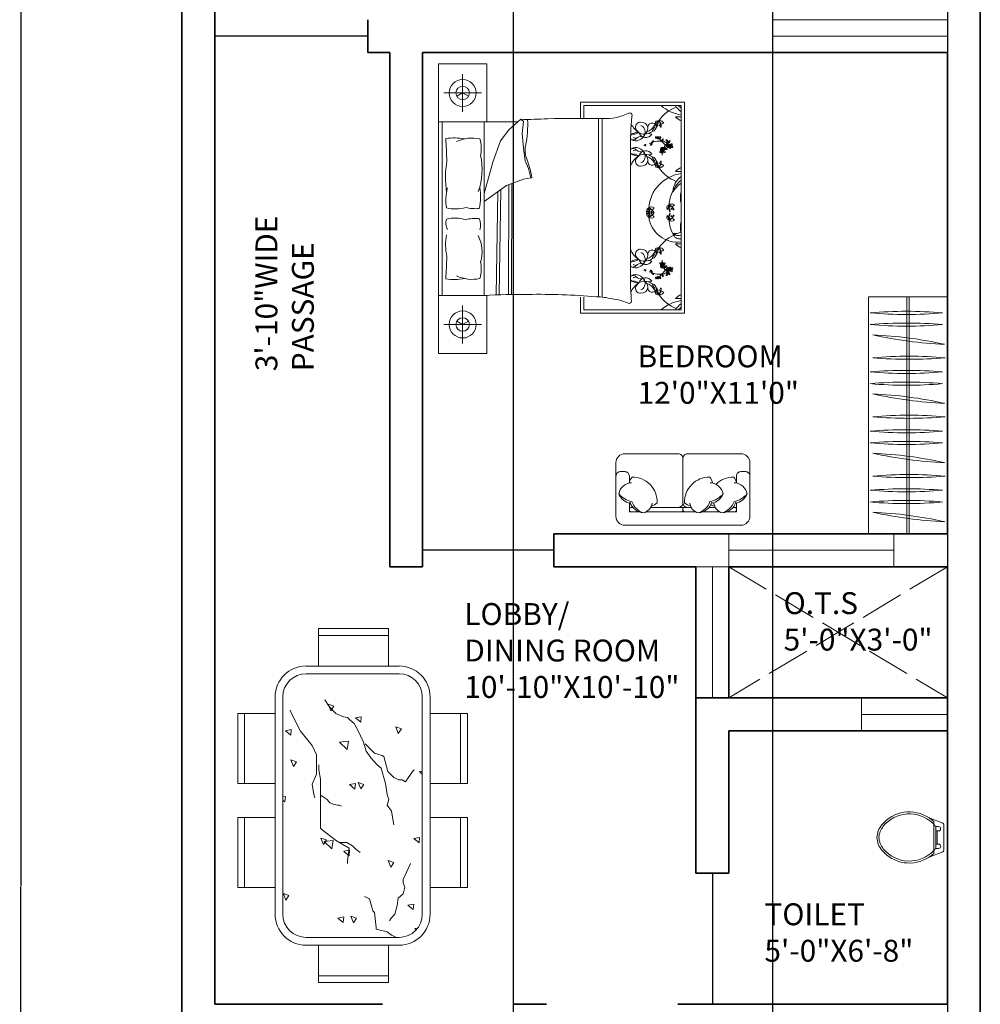
# Model space of a CAD drawing. Units: inches. Extents: x -16 to 587, y -783 to 64.
# Tile 13 of 14: x 279 to 543, y -392 to -122. Entities that reach past the tile are written whole.
import ezdxf

# ---------------------------------------------------------------- set-up
doc = ezdxf.new("R2010")
doc.units = ezdxf.units.IN
doc.header["$MEASUREMENT"] = 0
doc.linetypes.add('ACAD_ISO02W100', pattern=[15, 12, -3])
for name, color, linetype, lineweight in [('A-ANNO-DIMS', 2, 'Continuous', 18), ('A-AREA-IDEN', 7, 'Continuous', 18), ('A-DOOR', 3, 'Continuous', 25), ('A-FLOR-FIXT', 9, 'Continuous', 18), ('A-FLOR-OPEN', 8, 'ACAD_ISO02W100', 13), ('A-FURN', 8, 'Continuous', 18), ('A-GLAZ', 4, 'Continuous', 18), ('A-WALL', 7, 'Continuous', 35)]:
    doc.layers.add(name, color=color, linetype=linetype, lineweight=lineweight)
doc.styles.get("Standard").update_dxf_attribs({"font": 'arial.ttf'})
doc.dimstyles.get("Standard").update_dxf_attribs({"dimtxt": 0.18, "dimasz": 0.18, "dimexe": 0.18, "dimexo": 0.0625, "dimgap": 0.09, "dimtad": 0, "dimtih": 1, "dimtoh": 1, "dimdec": 0, "dimzin": 0, "dimdsep": 46, "dimlunit": 3, "dimtxsty": 'Standard', "dimcen": 0.09, "dimadec": 0, "dimazin": 0, "dimtfac": 1, "dimtdec": 0, "dimtofl": 0, "dimtmove": 0, "dimatfit": 3, "dimfxl": 1, "dimtolj": 1, "dimtzin": 0, "dimarcsym": 0})

# ---------------------------------------------------------------- blocks, each defined once
blk = doc.blocks.new('BED-DOUBLE-COMPACT')
for p, q in [((0, 79.37), (0, 0)), ((6.61, 66.25), (6.61, 76.62)), ((11.8, 71.43), (1.43, 71.43)), ((38.91, 68.89), (38.91, 64.4)), ((67.5, 68.89), (38.91, 68.89)), ((39.83, 64.41), (39.83, 67.97)), ((39.83, 67.97), (66.58, 67.97)), ((66.58, 67.97), (66.58, 11.95)), ((67.5, 11.03), (67.5, 68.89)), ((0, 63.5), (21.78, 63.5)), ((1.02, 15.87), (1.02, 63.5)), ((12.54, 63.5), (12.54, 15.87)), ((22.61, 64.21), (19.24, 61.31)), ((23.26, 63.56), (22.61, 64.21)), ((22.93, 60.35), (23.26, 63.56)), ((43.86, 15.51), (43.86, 64.41)), ((44.85, 15.44), (44.85, 64.41)), ((19.24, 61.31), (16.99, 58.26)), ((23.26, 56.33), (22.93, 60.35)), ((58.53, 60.15), (57.63, 60.33)), ((16.99, 58.26), (14.9, 52.47)), ((23.74, 52.79), (23.26, 56.33)), ((52.64, 23.57), (52.64, 55.8)), ((58.53, 54.61), (57.63, 54.43)), ((14.9, 52.47), (12.54, 43.82)), ((24.7, 50.7), (23.74, 52.79)), ((25.34, 48.13), (24.7, 50.7)), ((12.54, 41.69), (18.6, 46.04)), ((18.6, 46.04), (23.26, 47.81)), ((19.15, 16.16), (19.27, 46.3)), ((19.97, 16.15), (20.09, 46.61)), ((23.26, 47.81), (25.34, 48.13)), ((15.84, 16.09), (16.24, 44.34)), ((16.65, 16.12), (17.06, 44.94)), ((58.53, 25.32), (57.63, 25.49)), ((58.53, 19.77), (57.63, 19.6)), ((38.91, 15.43), (38.91, 11.03)), ((39.83, 11.95), (39.83, 15.45)), ((6.61, 13.12), (6.61, 2.75)), ((38.91, 11.03), (67.5, 11.03)), ((66.58, 11.95), (39.83, 11.95)), ((11.8, 7.94), (1.43, 7.94))]:
    blk.add_line(p, q)
for points in [[(13.23, 63.5), (13.23, 79.37), (0, 79.37)], [(6.61, 71.43), (5.01, 70.51)], [(6.61, 71.43), (8.22, 70.51)], [(0, 15.87), (13.23, 15.87), (13.23, 0), (0, 0)], [(6.61, 7.94), (5.01, 8.86)], [(6.61, 7.94), (8.22, 8.86)]]:
    blk.add_lwpolyline(points)
for points in [[(29.88, 64.37, -0.001242), (44.94, 64.41, 0.127202), (52.44, 66)], [(1.98, 58.94, -0.074897), (7.16, 58.84, 0.472817)], [(7.45, 40.06, -0.14099), (2.16, 39.9, -0.235245)], [(7.45, 36.67, 0.14099), (2.16, 36.83, 0.235245)], [(1.98, 20.43, 0.074897), (7.16, 20.53, -0.472817)], [(43.23, 15.54, -0.056112), (47.6, 14.96, -0.095341), (51.8, 13.84)]]:
    blk.add_lwpolyline(points, format="xyb")
for centre, radius in [((6.61, 71.43), 3.7), ((6.61, 71.43), 1.85), ((63.54, 56.89), 0.202), ((61.41, 55.57), 0.202), ((61.41, 24.36), 0.202), ((63.54, 23.03), 0.202), ((6.61, 7.94), 3.7), ((6.61, 7.94), 1.85)]:
    blk.add_circle(centre, radius)
for centre, radius, start, end in [((69, 57.96), 10.36, 111.4092, 145.6135), ((67.97, 75.69), 10.36, 228.1144, 262.255), ((69.36, 70.49), 5.05, 209.8884, 236.5383), ((70.3, 72.31), 6.29, 223.5186, 233.6964), ((52.39, 65.27), 0.732, 332.6588, 86.02), ((135.26, 56.74), 82.62, 174.3113, 180.6567), ((68.19, 67.66), 4.21, 221.0454, 247.4453), ((65.93, 79.2), 14.34, 266.3481, 272.5919), ((24.59, 136.98), 72.8, 268.447, 274.1706), ((-5.49, 62.85), 29.95, 348.6608, 2.5481), ((58.23, 65.58), 6.01, 206.7003, 236.3329), ((55.35, 62.08), 1.34, 88.9462, 185.5144), ((55.54, 61.53), 1.9, 7.1143, 95.0551), ((54.82, 60.79), 1.84, 338.5779, 68.4181), ((55.97, 64.33), 3.75, 288.2955, 328.7386), ((58.6, 61.97), 1.19, 19.1312, 189.736), ((58.24, 62.25), 1.49, 285.6955, 4.031), ((59.89, 62.21), 0.73, 126.7319, 206.0245), ((60.24, 62.98), 0.859, 76.272, 177.0484), ((58.93, 64.73), 1.77, 284.7031, 328.6173), ((61.4, 62.48), 1.64, 125.7657, 194.5347), ((53.37, 65.38), 7.25, 332.8176, 347.4827), ((60.69, 62.69), 1.15, 20.9613, 102.2885), ((61.31, 63.84), 0.866, 181.7131, 301.5367), ((58.47, 62.09), 2.62, 2.0648, 41.1598), ((60.05, 63.06), 0.848, 316.2238, 62.3173), ((60.58, 62.55), 0.112, 20.2817, 316.2238), ((60.96, 62.18), 0.129, 168.5166, 2.0648), ((60.9, 62.19), 0.0625, 52.0591, 168.5166), ((53.52, 59.3), 0.956, 127.675, 149.9707), ((53.23, 63.38), 3.29, 260.8446, 301.1782), ((54.08, 60.83), 2.53, 240.8249, 340.7178), ((54.66, 57.53), 3.06, 85.2696, 124.215), ((56.34, 62.49), 2.39, 193.079, 274.7067), ((55.44, 57.84), 1.63, 74.8529, 138.4347), ((56.82, 61.14), 1.97, 196.8663, 330.0915), ((55.99, 59.89), 0.493, 254.8529, 12.6959), ((54.66, 57.53), 3.06, 53.6555, 57.2989), ((55.12, 61.86), 2.31, 305.9599, 357.6409), ((56.28, 64.36), 4.26, 273.4924, 303.7117), ((60.21, 60.65), 1.58, 128.4175, 173.8338), ((59.89, 59.21), 0.337, 127.3642, 168.4363), ((60.01, 59.25), 0.193, 88.1325, 178.8919), ((60.21, 59.49), 0.202, 183.2768, 356.7232), ((60.14, 58.85), 0.614, 42.3896, 66.5724), ((60.58, 59.21), 0.334, 10.9597, 52.2379), ((-753.35, 15.19), 756.59, 2.85022, 3.31479), ((9.24, 48.82), 10.23, 78.2417, 114.8684), ((1.05, 56.11), 10.64, 348.9631, 14.8961), ((30.21, 55.69), 6.46, 168.6608, 203.7384), ((53.52, 59.3), 0.956, 206.442, 225.5483), ((53.33, 59.71), 1.19, 246.1646, 318.4347), ((54.54, 61.21), 2.28, 240.0851, 262.564), ((56.64, 57.17), 0.249, 169.5864, 349.5616), ((56.74, 57.15), 0.153, 349.5616, 167.2949), ((60.73, 51.65), 6.57, 110.1059, 116.9968), ((58.53, 57.07), 0.417, 129.5056, 182.6421), ((57.33, 58.03), 1.25, 308.4388, 328.836), ((57.11, 59.05), 2.24, 296.5064, 305.3102), ((57.1, 57.9), 1.28, 336.3901, 344.4871), ((58.48, 57.57), 0.162, 83.9457, 185.6216), ((57.84, 57.73), 0.665, 328.836, 0.8141), ((58.18, 57.53), 0.381, 306.5232, 32.4668), ((58.64, 57.83), 0.162, 112.5583, 214.2343), ((58.53, 58.12), 0.381, 265.7131, 351.6568), ((58.2, 58.33), 0.665, 297.3659, 329.344), ((57.69, 58.9), 1.28, 313.6929, 321.7899), ((59.1, 58.03), 0.417, 115.5379, 168.6744), ((57.69, 58.63), 1.25, 329.344, 349.7412), ((60.73, 51.65), 6.57, 86.1723, 106.4158), ((56.69, 58.34), 2.24, 352.8698, 1.6736), ((59.65, 59.15), 0.156, 125.0752, 284.7644), ((59.63, 59.48), 0.486, 277.4968, 341.2737), ((60.4, 59.04), 0.418, 136.3462, 189.6513), ((60.16, 59), 0.174, 189.6513, 312.3208), ((60.84, 59.12), 0.662, 164.2829, 186.9148), ((60.06, 59.12), 0.331, 312.3208, 40.2111), ((60.76, 59.49), 0.47, 201.6382, 274.947), ((66.33, 63.71), 7.54, 217.9541, 226.8459), ((60.79, 59.18), 0.155, 274.947, 37.5263), ((61.31, 58.3), 0.162, 112.5583, 214.2343), ((61.2, 58.59), 0.381, 265.7131, 351.6568), ((60.87, 58.8), 0.665, 297.3659, 329.344), ((60.9, 54.92), 3.3, 60.7959, 85.244), ((53.88, 50.18), 10.84, 37.8256, 47.7588), ((60.36, 59.37), 1.28, 313.6929, 321.7899), ((61.77, 58.5), 0.417, 115.5379, 168.6744), ((60.36, 59.1), 1.25, 329.344, 349.7412), ((59.36, 58.81), 2.24, 352.8698, 1.6736), ((65.28, 54.59), 3.95, 130.182, 149.456), ((62.5, 58.36), 0.226, 33.0979, 123.1364), ((57.53, 55.18), 5.91, 31.1156, 34.8118), ((62.18, 57.97), 0.611, 2.3172, 70.5201), ((63.1, 56.84), 0.652, 139.3812, 199.9959), ((61.88, 57.31), 0.921, 310.9365, 22.7695), ((62.31, 57.26), 0.669, 285.6484, 332.2957), ((62.68, 57.82), 0.176, 135.7354, 318.1297), ((62.39, 58.11), 0.234, 315.7354, 31.1156), ((62.19, 57.61), 0.542, 319.3812, 5.5456), ((62.81, 57.82), 0.176, 68.2452, 250.6395), ((62.41, 58.04), 0.526, 352.6008, 57.1845), ((64.29, 54.51), 3.52, 111.7087, 116.2181), ((60.9, 54.92), 3.3, 47.5083, 55.9967), ((62.91, 58.16), 0.526, 252.8042, 349.6943), ((62.41, 57.22), 0.56, 331.1838, 51.6792), ((62.97, 58.2), 0.234, 248.2452, 323.6254), ((63.22, 56.61), 0.337, 93.635, 168.4363), ((63.18, 57.14), 0.198, 138.2946, 276.2474), ((62.76, 58.35), 0.611, 291.7087, 3.0299), ((62.96, 56.88), 0.486, 277.4968, 341.2737), ((63.26, 57.11), 0.276, 358.5719, 143.8954), ((58.4, 61.57), 5.91, 323.6254, 327.3216), ((63.35, 56.65), 0.193, 88.1325, 178.8919), ((63.42, 57.33), 0.278, 208.8493, 269.9355), ((63.18, 57.26), 0.318, 274.2123, 318.1587), ((63.73, 56.45), 0.418, 136.3462, 189.6513), ((63.24, 58.19), 0.226, 325.6077, 55.6462), ((64.17, 56.53), 0.662, 164.2829, 186.9148), ((64.15, 56.94), 0.637, 121.9501, 165.2442), ((63.39, 56.52), 0.331, 312.3208, 40.2111), ((64.09, 56.9), 0.47, 201.6382, 274.947), ((63.71, 57.19), 0.134, 262.868, 7.094), ((63.47, 56.25), 0.614, 42.3896, 66.5724), ((63.69, 57.3), 0.399, 278.5614, 22.5914), ((63.91, 56.61), 0.334, 10.9597, 118.7804), ((63.92, 57.31), 0.2, 44.3732, 121.9501), ((-6.51, 50.51), 18.45, 340.7385, 11.9603), ((53.52, 55.45), 0.956, 134.4517, 156.771), ((53.52, 55.45), 0.956, 203.2856, 232.325), ((53.23, 51.38), 3.29, 58.8218, 100.2867), ((58.23, 49.18), 6.01, 123.6671, 158.5059), ((54.08, 53.93), 2.53, 19.2822, 119.1751), ((53.33, 55.05), 1.19, 41.5653, 113.8354), ((54.66, 57.23), 3.06, 235.785, 274.7304), ((54.54, 53.55), 2.28, 97.436, 119.9149), ((56.34, 52.27), 2.39, 85.2933, 166.921), ((55.44, 56.92), 1.63, 221.5653, 285.1471), ((56.82, 53.62), 1.97, 29.9085, 163.1337), ((54.82, 53.97), 1.84, 291.5819, 21.4221), ((55.99, 54.87), 0.493, 347.3041, 105.1471), ((54.66, 57.23), 3.06, 302.7011, 306.3445), ((55.12, 52.9), 2.31, 2.3591, 54.0401), ((56.28, 50.39), 4.26, 56.2883, 86.5076), ((60.85, 55.23), 0.156, 125.0752, 284.7644), ((61.09, 55.29), 0.337, 93.635, 168.4363), ((61.11, 57.11), 0.921, 253.6301, 325.4631), ((61.37, 55.83), 0.652, 82.0748, 142.6895), ((61.29, 56.73), 0.669, 228.342, 274.9894), ((61.05, 55.82), 0.198, 138.2946, 276.2474), ((60.83, 55.56), 0.486, 277.4968, 341.2737), ((61.13, 55.79), 0.276, 358.5719, 143.8954), ((61.22, 55.33), 0.193, 88.1325, 178.8919), ((61.29, 56.01), 0.278, 208.8493, 269.9355), ((61.05, 55.94), 0.318, 274.2123, 318.1587), ((61.6, 55.13), 0.418, 136.3462, 189.6513), ((61.36, 55.09), 0.174, 189.6513, 312.3208), ((65.28, 54.59), 3.95, 175.2415, 182.8929), ((61.31, 56.62), 0.56, 273.8774, 357.1501), ((62.04, 55.21), 0.662, 164.2829, 186.9148), ((62.02, 55.62), 0.637, 121.9501, 165.2442), ((61.53, 57.02), 0.542, 262.0748, 308.2393), ((61.26, 55.2), 0.331, 312.3208, 40.2111), ((61.96, 55.57), 0.47, 201.6382, 274.947), ((61.58, 55.87), 0.134, 262.868, 7.094), ((61.34, 54.93), 0.614, 42.3896, 66.5724), ((61.56, 55.98), 0.399, 278.5614, 22.5914), ((61.78, 55.29), 0.334, 10.9597, 118.7804), ((65.28, 54.59), 3.95, 156.1523, 156.9499), ((61.79, 55.99), 0.2, 44.3732, 121.9501), ((62.4, 56.46), 0.56, 181.4625, 249.4747), ((62.31, 56.9), 0.542, 215.1128, 261.2773), ((62.74, 56.87), 0.921, 197.889, 269.722), ((61.99, 55.26), 0.155, 274.947, 37.5263), ((62.46, 56.56), 0.669, 248.3627, 295.0101), ((62.13, 55.72), 0.652, 20.6625, 81.2773), ((62.98, 56.55), 0.156, 125.0752, 284.7644), ((63.49, 56.41), 0.174, 189.6513, 312.3208), ((64.12, 56.58), 0.155, 274.947, 37.5263), ((30.7, 48.06), 28.79, 170.503, 187.7804), ((-4.65, 42.62), 30.78, 10.6617, 19.8806), ((55.35, 52.68), 1.34, 174.4856, 271.0538), ((55.54, 53.23), 1.9, 264.9449, 352.8857), ((55.97, 50.43), 3.75, 31.2614, 71.7045), ((58.6, 52.79), 1.19, 170.264, 340.8688), ((60.21, 54.11), 1.58, 186.1662, 231.5825), ((58.24, 52.5), 1.49, 355.969, 74.3045), ((59.89, 52.54), 0.73, 153.9755, 233.2681), ((60.24, 51.78), 0.859, 182.9516, 283.728), ((58.93, 50.02), 1.77, 31.3827, 75.2969), ((61.4, 52.28), 1.64, 165.4653, 234.2343), ((53.37, 49.37), 7.25, 12.5173, 27.1824), ((58.47, 52.67), 2.62, 318.8402, 357.9352), ((60.05, 51.7), 0.848, 297.6827, 43.7762), ((61.31, 50.92), 0.866, 58.4633, 178.2869), ((60.69, 52.07), 1.15, 257.7115, 339.0387), ((60.54, 52.19), 0.0676, 43.7729, 339.7333), ((60.96, 52.58), 0.129, 357.9352, 191.4834), ((60.9, 52.57), 0.0625, 191.4834, 307.9409), ((67.97, 39.07), 10.36, 97.745, 175.5377), ((69, 56.8), 10.36, 214.3865, 248.5908), ((68.19, 47.1), 4.21, 112.5547, 138.9546), ((65.93, 35.55), 14.34, 87.4081, 93.6519), ((25.41, 48.31), 0.192, 250.2464, 1.1377), ((69.36, 44.27), 5.05, 123.4617, 178.728), ((70.3, 42.45), 6.29, 126.3036, 162.1496), ((72.07, 39.14), 9.36, 125.947, 145.9877), ((16.15, 41.98), 14.14, 166.04, 188.4751), ((-2.48, 43.04), 14, 346.3762, 10.1383), ((73.53, 39.86), 10.36, 152.5854, 175.5377), ((72.03, 42.76), 5.7, 162.9798, 196.4569), ((63.43, 39.84), 0.859, 106.1963, 206.9726), ((61.42, 40.71), 1.77, 314.6273, 358.5415), ((64.69, 39.99), 1.64, 155.6899, 224.4589), ((63.97, 39.82), 1.15, 50.8855, 132.2127), ((63.93, 41.12), 0.866, 211.6373, 331.4609), ((62.34, 38.19), 2.62, 31.989, 71.0841), ((56.27, 38.5), 7.25, 2.7418, 17.407), ((63.23, 39.82), 0.848, 346.148, 92.2415), ((74.96, 40.5), 8.43, 174.3643, 175.6213), ((80.74, 36.06), 15.06, 160.0972, 160.2783), ((10.1, 49.41), 9.72, 254.1707, 275.9871), ((57.88, 39.05), 0.859, 106.1963, 206.9726), ((57.88, 38.23), 0.859, 153.0274, 253.8037), ((55.87, 39.92), 1.77, 314.6273, 358.5415), ((55.87, 37.36), 1.77, 1.4585, 45.3727), ((59.14, 39.2), 1.64, 155.6899, 224.4589), ((59.14, 38.08), 1.64, 135.5411, 204.3101), ((58.41, 39.02), 1.15, 50.8855, 132.2127), ((58.38, 40.33), 0.866, 211.6373, 331.4609), ((50.72, 37.7), 7.25, 2.7418, 17.407), ((57.67, 39.03), 0.848, 346.148, 92.2415), ((56.79, 37.39), 2.62, 31.989, 71.0841), ((50.72, 39.57), 7.25, 342.593, 357.2582), ((56.79, 39.88), 2.62, 288.9159, 328.011), ((57.67, 38.25), 0.848, 267.7585, 13.852), ((58.38, 36.95), 0.866, 28.5391, 148.3627), ((58.39, 38.85), 0.112, 50.0755, 346.148), ((58.35, 38.44), 0.0676, 13.9791, 309.8091), ((58.91, 38.71), 0.129, 198.4408, 31.989), ((58.84, 38.69), 0.0625, 81.9833, 198.4408), ((58.91, 38.56), 0.129, 328.011, 161.5592), ((58.84, 38.58), 0.0625, 161.5592, 278.0167), ((63.43, 37.44), 0.859, 153.0274, 253.8037), ((61.42, 36.56), 1.77, 1.4585, 45.3727), ((64.69, 37.28), 1.64, 135.5411, 204.3101), ((56.27, 38.78), 7.25, 342.593, 357.2582), ((63.94, 39.64), 0.112, 50.0755, 346.148), ((64.39, 39.49), 0.0625, 81.9833, 198.4408), ((64.39, 37.79), 0.0625, 161.5592, 278.0167), ((64.46, 39.51), 0.129, 198.4408, 31.989), ((64.46, 37.77), 0.129, 328.011, 161.5592), ((5.94, 35.74), 3.93, 163.8974, 206.6563), ((10.1, 27.31), 9.72, 84.0129, 105.8293), ((7.31, 35.21), 4.21, 341.4593, 24.9817), ((58.41, 38.25), 1.15, 227.7873, 309.1145), ((65.58, 38.54), 8.02, 188.1803, 277.1364), ((62.34, 39.09), 2.62, 288.9159, 328.011), ((63.23, 37.46), 0.848, 267.7585, 13.852), ((63.93, 36.16), 0.866, 28.5391, 148.3627), ((63.97, 37.46), 1.15, 227.7873, 309.1145), ((73.53, 37.42), 10.36, 184.4623, 207.4146), ((63.9, 37.64), 0.0676, 13.9791, 309.8091), ((72.03, 34.52), 5.7, 163.5431, 197.0202), ((74.96, 36.78), 8.43, 184.3787, 185.6357), ((80.74, 41.21), 15.06, 199.7217, 199.9028), ((15.87, 29.85), 13.95, 168.8159, 193.6573), ((69, 23.12), 10.36, 111.4092, 145.6135), ((64.85, 37.51), 4.64, 263.3805, 291.883), ((66.14, 33.25), 1.86, 190.9261, 283.6102), ((65.88, 34.65), 2.35, 228.0951, 287.1391), ((1.83, 27.85), 10.1, 343.8254, 26.1239), ((65.93, 44.37), 14.34, 266.3481, 272.5919), ((68.19, 32.83), 4.21, 221.0454, 247.4453), ((58.23, 30.75), 6.01, 201.4941, 236.3329), ((55.35, 27.25), 1.34, 88.9462, 185.5144), ((56.34, 27.66), 2.39, 193.079, 274.7067), ((55.54, 26.7), 1.9, 7.1143, 95.0551), ((54.82, 25.95), 1.84, 338.5779, 68.4181), ((55.97, 29.5), 3.75, 288.2955, 328.7386), ((58.6, 27.13), 1.19, 19.1312, 189.736), ((58.24, 27.42), 1.49, 285.6955, 4.031), ((60.21, 25.82), 1.58, 128.4175, 173.8338), ((59.89, 27.38), 0.73, 126.7319, 206.0245), ((60.24, 28.14), 0.859, 76.272, 177.0484), ((58.93, 29.9), 1.77, 284.7031, 328.6173), ((61.4, 27.65), 1.64, 125.7657, 194.5347), ((53.37, 30.55), 7.25, 332.8176, 347.4827), ((60.69, 27.85), 1.15, 20.9613, 102.2885), ((60.05, 28.23), 0.848, 316.2238, 62.3173), ((58.47, 27.25), 2.62, 2.0648, 41.1598), ((61.31, 29), 0.866, 181.7131, 301.5367), ((60.58, 27.72), 0.112, 20.2817, 316.2238), ((60.96, 27.34), 0.129, 168.5166, 2.0648), ((60.9, 27.35), 0.0625, 52.0591, 168.5166), ((-753.35, 64.18), 756.59, 356.68521, 357.14978), ((1.05, 23.26), 10.64, 345.1039, 11.0369), ((53.23, 28.54), 3.29, 259.7133, 301.1782), ((53.52, 24.47), 0.956, 127.675, 156.7144), ((54.08, 26), 2.53, 240.8249, 340.7178), ((54.66, 22.7), 3.06, 85.2696, 124.215), ((54.54, 26.38), 2.28, 240.0851, 262.564), ((55.44, 23.01), 1.63, 74.8529, 138.4347), ((56.82, 26.3), 1.97, 196.8663, 330.0915), ((55.99, 25.05), 0.493, 254.8529, 12.6959), ((54.66, 22.7), 3.06, 53.6555, 57.2989), ((55.12, 27.03), 2.31, 305.9599, 357.6409), ((56.28, 29.53), 4.26, 273.4924, 303.7117), ((60.85, 24.7), 0.156, 75.2356, 234.9248), ((61.09, 24.64), 0.337, 191.5637, 266.365), ((61.05, 24.1), 0.198, 83.7526, 221.7054), ((60.83, 24.37), 0.486, 18.7263, 82.5032), ((61.22, 24.59), 0.193, 181.1081, 271.8675), ((61.36, 24.84), 0.174, 47.6792, 170.3487), ((61.6, 24.8), 0.418, 170.3487, 223.6538), ((65.28, 25.34), 3.95, 177.1071, 184.7585), ((62.04, 24.72), 0.662, 173.0852, 195.7171), ((61.26, 24.72), 0.331, 319.7889, 47.6792), ((61.96, 24.35), 0.47, 85.053, 158.3618), ((61.34, 24.99), 0.614, 293.4276, 317.6104), ((61.78, 24.63), 0.334, 241.2196, 349.0403), ((61.56, 23.94), 0.399, 337.4086, 81.4386), ((61.99, 24.66), 0.155, 322.4737, 85.053), ((129.84, 21.14), 77.23, 178.1965, 184.7598), ((53.52, 24.47), 0.956, 203.2856, 225.5483), ((53.33, 24.87), 1.19, 246.1646, 318.4347), ((54.08, 19.09), 2.53, 19.2822, 119.1751), ((56.64, 22.76), 0.249, 10.4384, 190.4136), ((56.74, 22.77), 0.153, 192.7051, 10.4384), ((60.73, 28.27), 6.57, 243.0032, 249.8941), ((57.33, 21.89), 1.25, 31.164, 51.5612), ((58.53, 22.86), 0.417, 177.3579, 230.4944), ((57.11, 20.87), 2.24, 54.6898, 63.4936), ((57.1, 22.02), 1.28, 15.5129, 23.6099), ((58.48, 22.35), 0.162, 174.3784, 276.0543), ((58.18, 22.39), 0.381, 327.5332, 53.4768), ((57.84, 22.2), 0.665, 359.1859, 31.164), ((58.64, 22.1), 0.162, 145.7657, 247.4417), ((58.53, 21.81), 0.381, 8.3432, 94.2869), ((58.2, 21.6), 0.665, 30.656, 62.6341), ((57.69, 21.03), 1.28, 38.2101, 46.3071), ((59.1, 21.9), 0.417, 191.3256, 244.4621), ((57.69, 21.3), 1.25, 10.2588, 30.656), ((60.73, 28.27), 6.57, 253.5842, 273.8277), ((56.69, 21.59), 2.24, 358.3264, 7.1302), ((66.33, 16.22), 7.54, 133.1541, 142.0459), ((61.29, 23.19), 0.669, 85.0106, 131.658), ((61.11, 22.81), 0.921, 34.5369, 106.3699), ((61.37, 24.09), 0.652, 217.3105, 277.9252), ((61.13, 24.13), 0.276, 216.1046, 1.4281), ((61.29, 23.92), 0.278, 90.0645, 151.1507), ((61.05, 23.98), 0.318, 41.8413, 85.7877), ((61.31, 21.62), 0.162, 145.7657, 247.4417), ((53.88, 29.74), 10.84, 312.2412, 322.1744), ((60.9, 25), 3.3, 274.756, 299.2041), ((61.2, 21.33), 0.381, 8.3432, 94.2869), ((60.87, 21.12), 0.665, 30.656, 62.6341), ((61.31, 23.3), 0.56, 2.8499, 86.1226), ((62.02, 24.3), 0.637, 194.7558, 238.0499), ((61.53, 22.91), 0.542, 51.7607, 97.9252), ((61.58, 24.06), 0.134, 352.906, 97.132), ((65.28, 25.34), 3.95, 203.0501, 203.8477), ((61.79, 23.93), 0.2, 238.0499, 315.6268), ((62.4, 23.46), 0.56, 110.5253, 178.5375), ((62.74, 23.05), 0.921, 90.278, 162.111), ((62.31, 23.02), 0.542, 98.7227, 144.8872), ((65.28, 25.34), 3.95, 210.544, 229.818), ((62.46, 23.36), 0.669, 64.9899, 111.6373), ((62.13, 24.2), 0.652, 278.7227, 339.3375), ((62.18, 21.95), 0.611, 289.4799, 357.6828), ((57.53, 24.75), 5.91, 325.1882, 328.8844), ((63.1, 23.09), 0.652, 160.0041, 220.6188), ((61.88, 22.61), 0.921, 337.2305, 49.0635), ((62.31, 22.66), 0.669, 27.7043, 74.3516), ((62.68, 22.1), 0.176, 41.8703, 224.2646), ((62.39, 21.82), 0.234, 328.8844, 44.2646), ((62.19, 22.31), 0.542, 354.4544, 40.6188), ((62.81, 22.1), 0.176, 109.3605, 291.7548), ((62.41, 21.88), 0.526, 302.8155, 7.3992), ((64.29, 25.42), 3.52, 243.7819, 248.2913), ((60.9, 25), 3.3, 304.0033, 312.4917), ((62.41, 22.71), 0.56, 308.3208, 28.8162), ((62.91, 21.76), 0.526, 10.3057, 107.1958), ((62.98, 23.37), 0.156, 75.2356, 234.9248), ((62.97, 21.72), 0.234, 36.3746, 111.7548), ((63.22, 23.31), 0.337, 191.5637, 266.365), ((63.18, 22.78), 0.198, 83.7526, 221.7054), ((62.76, 21.58), 0.611, 356.9701, 68.2913), ((62.96, 23.04), 0.486, 18.7263, 82.5032), ((63.26, 22.81), 0.276, 216.1046, 1.4281), ((63.35, 23.27), 0.193, 181.1081, 271.8675), ((58.4, 18.36), 5.91, 32.6784, 36.3746), ((63.42, 22.59), 0.278, 90.0645, 151.1507), ((63.18, 22.66), 0.318, 41.8413, 85.7877), ((63.49, 23.52), 0.174, 47.6792, 170.3487), ((63.73, 23.47), 0.418, 170.3487, 223.6538), ((63.24, 21.73), 0.226, 304.3538, 34.3923), ((64.17, 23.4), 0.662, 173.0852, 195.7171), ((64.15, 22.98), 0.637, 194.7558, 238.0499), ((63.39, 23.4), 0.331, 319.7889, 47.6792), ((64.09, 23.03), 0.47, 85.053, 158.3618), ((63.71, 22.74), 0.134, 352.906, 97.132), ((63.47, 23.67), 0.614, 293.4276, 317.6104), ((63.91, 23.31), 0.334, 241.2196, 349.0403), ((63.69, 22.62), 0.399, 337.4086, 81.4386), ((63.92, 22.61), 0.2, 238.0499, 315.6268), ((64.12, 23.34), 0.155, 322.4737, 85.053), ((9.24, 30.54), 10.23, 245.1316, 281.7583), ((53.52, 20.62), 0.956, 134.4517, 163.3657), ((53.52, 20.62), 0.956, 197.4186, 232.325), ((53.23, 16.55), 3.29, 58.8218, 100.751), ((58.23, 14.34), 6.01, 123.6671, 156.3547), ((53.33, 20.22), 1.19, 41.5653, 113.8354), ((54.66, 22.39), 3.06, 235.785, 274.7304), ((54.54, 18.71), 2.28, 97.436, 119.9149), ((56.34, 17.43), 2.39, 85.2933, 166.921), ((55.44, 22.08), 1.63, 221.5653, 285.1471), ((56.82, 18.79), 1.97, 29.9085, 163.1337), ((54.82, 19.14), 1.84, 291.5819, 21.4221), ((55.99, 20.04), 0.493, 347.3041, 105.1471), ((54.66, 22.39), 3.06, 302.7011, 306.3445), ((55.12, 18.06), 2.31, 2.3591, 54.0401), ((56.28, 15.56), 4.26, 56.2883, 86.5076), ((55.97, 15.59), 3.75, 31.2614, 71.7045), ((58.24, 17.67), 1.49, 355.969, 74.3045), ((60.21, 19.27), 1.58, 186.1662, 231.5825), ((59.65, 20.78), 0.156, 75.2356, 234.9248), ((59.89, 20.72), 0.337, 191.5637, 232.6358), ((59.63, 20.45), 0.486, 18.7263, 82.5032), ((60.01, 20.67), 0.193, 181.1081, 271.8675), ((60.16, 20.92), 0.174, 47.6792, 170.3487), ((60.4, 20.88), 0.418, 170.3487, 223.6538), ((60.21, 20.44), 0.202, 3.2768, 176.7232), ((60.84, 20.8), 0.662, 173.0852, 195.7171), ((60.06, 20.8), 0.331, 319.7889, 47.6792), ((60.76, 20.43), 0.47, 85.053, 158.3618), ((60.14, 21.07), 0.614, 293.4276, 317.6104), ((60.58, 20.71), 0.334, 307.7621, 349.0403), ((60.79, 20.74), 0.155, 322.4737, 85.053), ((60.36, 20.55), 1.28, 38.2101, 46.3071), ((61.77, 21.42), 0.417, 191.3256, 244.4621), ((60.36, 20.82), 1.25, 10.2588, 30.656), ((59.36, 21.11), 2.24, 358.3264, 7.1302), ((62.5, 21.56), 0.226, 236.8636, 326.9021), ((22.24, -126.41), 142.61, 89.0718, 93.9), ((27.43, -169.82), 186.03, 85.1265, 90.8855), ((55.35, 17.84), 1.34, 174.4856, 271.0538), ((55.54, 18.39), 1.9, 264.9449, 352.8857), ((58.6, 17.96), 1.19, 170.264, 340.8688), ((59.89, 17.71), 0.73, 153.9755, 233.2681), ((58.93, 15.19), 1.77, 31.3827, 75.2969), ((60.24, 16.95), 0.859, 182.9516, 283.728), ((61.4, 17.44), 1.64, 165.4653, 234.2343), ((53.37, 14.54), 7.25, 12.5173, 27.1824), ((58.47, 17.84), 2.62, 318.8402, 357.9352), ((60.05, 16.86), 0.848, 297.6827, 43.7762), ((61.31, 16.09), 0.866, 58.4633, 178.2869), ((60.69, 17.24), 1.15, 257.7115, 339.0387), ((60.54, 17.36), 0.0676, 43.7729, 339.7333), ((60.96, 17.75), 0.129, 357.9352, 191.4834), ((60.9, 17.73), 0.0625, 191.4834, 307.9409), ((52.21, 14.44), 0.723, 236.1736, 23.4781), ((69, 21.97), 10.36, 214.3865, 248.5908), ((67.97, 4.23), 10.36, 97.745, 131.8856), ((69.36, 9.43), 5.05, 123.4617, 150.1116), ((68.19, 12.26), 4.21, 112.5547, 138.9546), ((65.93, 0.72), 14.34, 87.4081, 93.6519), ((70.3, 7.62), 6.29, 126.3036, 136.4814)]:
    blk.add_arc(centre, radius, start, end)
blk = doc.blocks.new('WARDROBE')
for p, q in [((0, 0), (0, 65.01)), ((21.67, 65.01), (0, 65.01)), ((10.47, 0), (10.47, 65.01)), ((11.19, 0), (11.19, 65.01)), ((21.67, 0), (21.67, 65.01)), ((21.67, 0), (0, 0))]:
    blk.add_line(p, q)
for centre, start, end in [((10.4, -52.98), 85.0028, 94.9972), ((10.4, 174.18), 265.0028, 274.9972), ((10.4, -56.19), 85.0028, 94.9972), ((10.4, 170.97), 265.0028, 274.9972), ((25.83, 165.89), 257.508, 267.5023), ((-3.8, -59.33), 77.508, 87.5023), ((11.1, -65.28), 85.0028, 94.9972), ((11.1, 161.88), 265.0028, 274.9972), ((10.4, -69.18), 85.0028, 94.9972), ((10.4, 157.98), 265.0028, 274.9972), ((10.4, -72.39), 85.0028, 94.9972), ((10.4, 154.77), 265.0028, 274.9972), ((25.83, 149.7), 257.508, 267.5023), ((-3.8, -75.52), 77.508, 87.5023), ((11.1, -81.47), 85.0028, 94.9972), ((11.1, 145.69), 265.0028, 274.9972), ((10.4, -85.44), 85.0028, 94.9972), ((10.4, 141.72), 265.0028, 274.9972), ((10.4, -88.65), 85.0028, 94.9972), ((10.4, 138.51), 265.0028, 274.9972), ((-3.8, -91.78), 77.508, 87.5023), ((25.83, 133.44), 257.508, 267.5023), ((11.1, -97.73), 85.0028, 94.9972), ((11.1, 129.43), 265.0028, 274.9972), ((10.4, -101.63), 85.0028, 94.9972), ((10.4, 125.53), 265.0028, 274.9972), ((10.4, -104.84), 85.0028, 94.9972), ((10.4, 122.32), 265.0028, 274.9972), ((-3.8, -107.97), 77.508, 87.5023), ((25.83, 117.25), 257.508, 267.5023)]:
    blk.add_arc(centre, 114.01, start, end)
blk = doc.blocks.new('DINING-TABLE-SIX')
for p, q in [((41.34, 97.05), (22.2, 97.05)), ((22.2, 97.05), (22.2, 86.8)), ((22.2, 95.18), (41.34, 95.18)), ((41.34, 86.8), (41.34, 97.05)), ((44.27, 86.8), (18.76, 86.8)), ((18.76, 84.68), (44.27, 84.68)), ((10.25, 78.3), (10.25, 18.76)), ((12.38, 18.76), (12.38, 78.3)), ((23.9, 77.51), (25.06, 75.66)), ((25.54, 74.52), (24.86, 76.31)), ((26.4, 75.79), (24.86, 76.31)), ((25.06, 75.66), (26.91, 73.81)), ((25.54, 74.52), (26.4, 75.79)), ((50.65, 78.3), (50.65, 18.76)), ((52.78, 18.76), (52.78, 78.3)), ((0, 54.61), (0, 73.75)), ((0, 73.75), (10.25, 73.75)), ((1.87, 73.75), (1.87, 54.61)), ((14.43, 74.74), (14.9, 73.58)), ((14.9, 73.58), (17.21, 68.96)), ((26.91, 73.81), (28.99, 72.89)), ((63.03, 73.75), (52.78, 73.75)), ((61.16, 73.75), (61.16, 54.61)), ((63.03, 54.61), (63.03, 73.75)), ((28.99, 72.89), (30.14, 72.66)), ((30.14, 72.66), (30.83, 71.96)), ((30.83, 71.96), (31.99, 71.04)), ((31.99, 71.04), (32.91, 69.42)), ((33.89, 72.89), (32.29, 72.59)), ((33.76, 71.36), (32.29, 72.59)), ((33.76, 71.36), (33.89, 72.89)), ((14.7, 69.35), (13.1, 69.05)), ((14.56, 67.82), (13.1, 69.05)), ((14.56, 67.82), (14.7, 69.35)), ((17.21, 68.96), (20.44, 65.03)), ((32.91, 69.42), (34.53, 65.95)), ((44.91, 69.58), (43.36, 70.1)), ((44.05, 68.31), (43.36, 70.1)), ((44.05, 68.31), (44.9, 69.58)), ((20.44, 65.03), (21.59, 62.48)), ((30.4, 66.21), (27.97, 65.93)), ((30.04, 63.94), (27.97, 65.93)), ((30.04, 63.94), (30.4, 66.21)), ((34.53, 65.95), (35.22, 63.41)), ((34.99, 65.49), (35.91, 64.56)), ((21.59, 62.48), (21.59, 57.16)), ((35.22, 63.41), (36.61, 61.56)), ((35.91, 64.56), (37.53, 62.94)), ((37.53, 62.94), (39.61, 62.25)), ((39.61, 62.25), (40.07, 62.02)), ((15.27, 59.29), (14.58, 61.08)), ((16.13, 60.56), (14.59, 61.08)), ((15.27, 59.29), (16.13, 60.56)), ((22.29, 59.71), (22.29, 58.32)), ((36.61, 61.56), (38.22, 59.71)), ((38.22, 59.71), (39.38, 58.78)), ((40.07, 62.02), (41.23, 57.86)), ((21.59, 57.16), (20.44, 54.39)), ((22.29, 58.32), (22.75, 55.78)), ((39.38, 58.78), (40.53, 54.62)), ((41.23, 57.86), (42.84, 56.24)), ((46.08, 55.08), (47.92, 57.86)), ((47.92, 57.86), (48.39, 58.32)), ((50.65, 57.18), (49.88, 57.83)), ((50.65, 57.97), (49.89, 57.83)), ((10.25, 54.61), (0, 54.61)), ((20.44, 54.39), (20.9, 51.61)), ((22.75, 55.78), (22.75, 42.37)), ((32.29, 54.58), (30.69, 54.29)), ((32.16, 53.06), (30.69, 54.29)), ((32.16, 53.06), (32.29, 54.58)), ((33.77, 53.08), (33.09, 54.87)), ((34.63, 54.35), (33.09, 54.87)), ((33.77, 53.08), (34.63, 54.35)), ((40.53, 54.62), (41, 51.61)), ((42.84, 56.24), (44.23, 55.55)), ((44.23, 55.55), (45.15, 55.55)), ((45.15, 55.55), (46.08, 55.08)), ((52.78, 54.61), (63.03, 54.61)), ((20.9, 51.61), (21.13, 50.69)), ((22.74, 51.39), (23.43, 50.92)), ((41, 51.61), (41.46, 50.23)), ((13.1, 51.04), (12.38, 50.91)), ((12.96, 49.52), (12.38, 50.01)), ((12.96, 49.52), (13.1, 51.04)), ((23.43, 50.92), (24.59, 50.23)), ((24.59, 50.23), (25.28, 49.31)), ((25.28, 49.31), (26.44, 48.84)), ((26.44, 48.84), (27.36, 48.61)), ((27.36, 48.61), (27.82, 48.61)), ((27.82, 48.61), (28.51, 48.38)), ((41.46, 50.23), (41, 48.61)), ((41, 48.61), (42.15, 46.99)), ((42.15, 46.99), (42.84, 43.29)), ((0, 26.11), (0, 45.25)), ((0, 45.25), (10.25, 45.25)), ((1.87, 45.25), (1.87, 26.11)), ((63.03, 45.25), (52.78, 45.25)), ((61.16, 45.25), (61.16, 26.11)), ((63.03, 26.11), (63.03, 45.25)), ((22.75, 42.37), (23.21, 41.9)), ((23.21, 41.9), (27.14, 38.9)), ((23.5, 37.85), (22.81, 39.64)), ((24.36, 39.12), (22.82, 39.64)), ((23.5, 37.85), (24.36, 39.12)), ((26.17, 38.97), (23.75, 38.69)), ((25.82, 36.7), (23.75, 38.69)), ((25.82, 36.7), (26.17, 38.97)), ((27.14, 38.9), (30.6, 36.82)), ((27.83, 38.43), (29.91, 38.43)), ((29.91, 38.43), (31.53, 37.51)), ((49.88, 39.82), (48.28, 39.53)), ((49.75, 38.3), (48.28, 39.53)), ((49.75, 38.3), (49.88, 39.82)), ((30.69, 36.28), (29.09, 35.99)), ((30.56, 34.75), (29.09, 35.98)), ((30.6, 36.82), (30.14, 33.35)), ((30.56, 34.75), (30.69, 36.28)), ((31.53, 37.51), (32.45, 36.58)), ((32.45, 36.58), (33.6, 35.66)), ((30.14, 33.35), (30.14, 32.65)), ((42.01, 31.64), (41.32, 33.43)), ((42.86, 32.91), (41.32, 33.43)), ((42.01, 31.64), (42.86, 32.91)), ((47.45, 32.66), (45.37, 28.26)), ((45.37, 28.26), (45.37, 27.34)), ((45.37, 27.34), (45.84, 26.18)), ((10.25, 26.11), (0, 26.11)), ((13.23, 22.62), (12.54, 24.41)), ((14.08, 23.89), (12.54, 24.41)), ((45.37, 24.33), (43.99, 23.18)), ((45.84, 26.18), (45.37, 24.33)), ((52.78, 26.11), (63.03, 26.11)), ((13.23, 22.62), (14.08, 23.89)), ((36.14, 22.94), (34.76, 23.64)), ((37.07, 19.7), (36.14, 22.94)), ((43.99, 23.18), (43.76, 21.1)), ((37.53, 19.24), (37.07, 19.7)), ((37.99, 15.08), (37.53, 19.24)), ((43.76, 21.1), (43.07, 18.78)), ((48.28, 21.52), (46.68, 21.22)), ((48.15, 19.99), (46.68, 21.22)), ((48.15, 19.99), (48.28, 21.52)), ((29.09, 17.98), (27.49, 17.68)), ((28.95, 16.45), (27.49, 17.68)), ((28.95, 16.45), (29.09, 17.98)), ((31.73, 16.41), (31.05, 18.2)), ((32.59, 17.68), (31.05, 18.2)), ((31.73, 16.41), (32.59, 17.68)), ((42.14, 17.63), (41.68, 16.93)), ((43.07, 18.78), (42.14, 17.63)), ((37.99, 14.62), (37.99, 15.08)), ((41, 13.92), (37.99, 14.62)), ((42.15, 13), (41, 13.92)), ((49.38, 14.93), (48.61, 14.84)), ((49, 14.47), (48.61, 14.84)), ((44.27, 12.38), (18.76, 12.38)), ((43.3, 12.54), (42.15, 13)), ((18.76, 10.25), (44.27, 10.25)), ((22.2, 10.25), (22.2, 0)), ((41.34, 0), (41.34, 10.25)), ((41.34, 1.87), (22.2, 1.87)), ((22.2, 0), (41.34, 0))]:
    blk.add_line(p, q)
for centre, radius, start, end in [((18.76, 78.3), 8.51, 90, 180), ((44.27, 78.3), 8.51, 0, 90), ((18.76, 78.3), 6.38, 90, 180), ((44.27, 78.3), 6.38, 0, 90), ((18.76, 18.76), 8.51, 180, 270), ((18.76, 18.76), 6.38, 180, 270), ((44.27, 18.76), 6.38, 270, 0), ((44.27, 18.76), 8.51, 270, 0)]:
    blk.add_arc(centre, radius, start, end)
blk = doc.blocks.new('WC-PLAN')
for p, q in [((15.58, 11.39), (15.58, 10.62)), ((15.58, 10.62), (15.58, 7.01)), ((15.58, 3.4), (15.58, 7.01)), ((15.58, 3.4), (15.58, 2.63))]:
    blk.add_line(p, q)
for points in [[(14.32, 12.39, 0.383919), (1.32, 10.46, 0.163732), (0, 7.01, 0.359733)], [(15.2, 10.99, 0.431639), (1.75, 10.11, 0.162618), (0.55, 7.01, 0.470877)], [(15.58, 11.39, 0.040937), (14.32, 12.39, 0.163732)], [(18.36, 7.01), (18.36, 10.52, 0.31031), (18.06, 10.95), (14.32, 12.39, 0.209071)], [(15.58, 10.62, 0.014165), (15.2, 10.99, 0.162618)], [(16.13, 9.99, 0.022712), (15.58, 10.62, 0.162618)], [(16.13, 7.01), (16.13, 9.99, 0.022712)], [(16.13, 9.99), (16.9, 9.99, -1), (16.9, 8.82), (16.5, 8.82)], [(14.32, 1.64, -0.383919), (1.32, 3.56, -0.163732), (0, 7.01, -0.359733)], [(15.58, 3.4, -0.448546), (1.75, 3.91, -0.162618), (0.55, 7.01, -0.470877)], [(18.36, 7.01), (18.36, 3.51, -0.31031), (18.06, 3.08), (14.32, 1.64, -0.209071)], [(16.13, 7.01), (16.13, 4.03, -0.476108)], [(16.13, 4.03, -0.022712), (15.58, 3.4, -0.162618)], [(16.13, 4.03), (16.9, 4.03, 1), (16.9, 5.21), (16.5, 5.21)], [(15.58, 2.63, -0.040937), (14.32, 1.64, -0.163732)]]:
    blk.add_lwpolyline(points, format="xyb")
for points in [[(16.5, 8.82), (16.13, 8.82)], [(16.5, 5.21), (16.5, 8.82)], [(16.5, 5.21), (16.13, 5.21)]]:
    blk.add_lwpolyline(points)
blk = doc.blocks.new('WIN-48')
for p, q in [((0, 9), (0, 0)), ((48, 9), (0, 9)), ((48, 0), (48, 9)), ((0, 4.5), (48, 4.5)), ((0, 0), (48, 0))]:
    blk.add_line(p, q)
blk = doc.blocks.new('*D53')
at = {"layer": 'A-ANNO-DIMS', "color": 0, "lineweight": -2, "transparency": 16777216}
for p, q in [((323.73, 19.45), (279.46, 19.45)), ((279.64, 19.27), (279.64, -358.87)), ((279.64, -737.37), (279.64, -359.24)), ((323.73, -737.55), (279.46, -737.55))]:
    blk.add_line(p, q, dxfattribs=at)
at = {"layer": 'A-ANNO-DIMS', "color": 0, "transparency": 16777216}
for points in [[(279.61, 19.27), (279.67, 19.27), (279.64, 19.45)], [(279.61, -737.37), (279.67, -737.37), (279.64, -737.55)]]:
    blk.add_solid(points, dxfattribs=at)
at = {"layer": 'Defpoints', "color": 0, "transparency": 16777216}
for p in [(323.79, 19.45), (279.64, -737.55), (323.79, -737.55)]:
    blk.add_point(p, dxfattribs=at)
at = {"layer": 'A-ANNO-DIMS', "color": 0, "transparency": 16777216, "insert": (279.64, -359.05), "char_height": 0.18, "attachment_point": 5}
blk.add_mtext('\\A1;63\'-1"', dxfattribs=at)
blk = doc.blocks.new('*D55')
at = {"layer": 'A-ANNO-DIMS', "color": 0, "lineweight": -2, "transparency": 16777216}
for p, q in [((485.79, -75.62), (485.79, -781.88)), ((533.79, -75.62), (533.79, -781.88)), ((485.97, -781.7), (509.46, -781.7)), ((533.61, -781.7), (510.12, -781.7))]:
    blk.add_line(p, q, dxfattribs=at)
at = {"layer": 'A-ANNO-DIMS', "color": 0, "transparency": 16777216}
for points in [[(485.97, -781.67), (485.97, -781.73), (485.79, -781.7)], [(533.61, -781.67), (533.61, -781.73), (533.79, -781.7)]]:
    blk.add_solid(points, dxfattribs=at)
at = {"layer": 'Defpoints', "color": 0, "transparency": 16777216}
for p in [(485.79, -75.55), (533.79, -75.55), (533.79, -781.7)]:
    blk.add_point(p, dxfattribs=at)
at = {"layer": 'A-ANNO-DIMS', "color": 0, "transparency": 16777216, "insert": (509.79, -781.7), "char_height": 0.18, "attachment_point": 5}
blk.add_mtext('\\A1;4\'-0"', dxfattribs=at)
blk = doc.blocks.new('*D59')
at = {"layer": 'A-ANNO-DIMS', "color": 0, "lineweight": -2, "transparency": 16777216}
for p, q in [((414.79, -712.99), (414.79, 63.78)), ((414.97, 63.6), (478.4, 63.6)), ((542.61, 63.6), (479.18, 63.6)), ((542.79, -712.99), (542.79, 63.78))]:
    blk.add_line(p, q, dxfattribs=at)
at = {"layer": 'A-ANNO-DIMS', "color": 0, "transparency": 16777216}
for points in [[(414.97, 63.63), (414.97, 63.57), (414.79, 63.6)], [(542.61, 63.63), (542.61, 63.57), (542.79, 63.6)]]:
    blk.add_solid(points, dxfattribs=at)
at = {"layer": 'Defpoints', "color": 0, "transparency": 16777216}
for p in [(542.79, 63.6), (414.79, -713.05), (542.79, -713.05)]:
    blk.add_point(p, dxfattribs=at)
at = {"layer": 'A-ANNO-DIMS', "color": 0, "transparency": 16777216, "insert": (478.79, 63.6), "char_height": 0.18, "attachment_point": 5}
blk.add_mtext('\\A1;10\'-8"', dxfattribs=at)

msp = doc.modelspace()

# ---------------------------------------------------------------- linework, layer by layer
at = {"layer": 'A-DOOR'}
for p, q in [((374.79, -126.05), (332.79, -126.05)), ((425.79, -267.05), (389.79, -267.05)), ((469.29, -355.55), (469.29, -391.55))]:
    msp.add_line(p, q, dxfattribs=at)
at = {"layer": 'A-FLOR-OPEN'}
for p, q in [((473.79, -271.55), (533.79, -307.55)), ((533.79, -271.55), (473.79, -307.55))]:
    msp.add_line(p, q, dxfattribs=at)
at = {"layer": 'A-FURN', "ltscale": 0.03}
msp.add_lwpolyline([(459.99, -240.57, -0.414214), (461.22, -241.8, -0.414214), (462.44, -240.57), (477.15, -240.57, -0.414214), (479.6, -243.03), (479.6, -257.73, -0.414214), (477.15, -260.18), (445.29, -260.18, -0.414214), (442.84, -257.73), (442.84, -243.03, -0.414214), (445.29, -240.57), (459.99, -240.57, -0.414214), (461.22, -241.8, -0.414214), (462.44, -240.57)], format="xyb", dxfattribs=at)
at = {"layer": 'A-FURN'}
for points in [[(459.99, -255.28, 0.414214), (461.22, -254.05), (461.22, -241.8, 0.414214)], [(462.44, -255.28, -0.414214), (461.22, -254.05), (461.22, -241.8, -0.414214)], [(442.84, -246.7, -0.414214), (444.07, -245.48), (445.29, -245.48, -0.414214), (446.52, -246.7), (446.52, -248.6)], [(475.92, -248.6), (475.92, -246.7, -0.414214), (477.15, -245.48), (478.37, -245.48, -0.414214), (479.6, -246.7)], [(446.51, -248.6, -0.165541), (447.27, -246.98, -0.425989), (454.15, -254, -0.121523), (452.52, -254.97, 7.115464)], [(469.32, -248.6, 0.165541), (468.57, -246.98, 0.425989), (461.68, -254, 0.121523), (463.32, -254.97, -7.115464)], [(475.92, -248.6, 0.165541), (475.17, -246.98, 0.200231), (470.3, -248.95, 0.121523)], [(447.13, -248.52, 0.356772), (443.62, -251.61, 0.249542), (446.8, -254.16, -9.61688)], [(468.71, -248.52, -0.356772), (472.22, -251.61, -0.249542), (469.04, -254.16, 9.61688)], [(475.31, -248.52, -0.356772), (478.82, -251.61, -0.249542), (475.64, -254.16, 9.61688)], [(443.62, -251.61, 0.14773), (447.2, -253.72, 0.213343), (450.36, -256.81, 0.178662)], [(472.22, -251.61, -0.14773), (468.64, -253.72, -0.213343), (465.48, -256.81, -0.178662)], [(478.82, -251.61, -0.14773), (475.24, -253.72, -0.213343), (472.08, -256.81, -0.178662)], [(447.45, -255.28), (447.01, -255.28, 0.414214), (446.52, -255.77), (446.52, -256.01, 0.414214), (447.01, -256.5)], [(446.71, -253.89, 0.306663), (450.36, -256.81, 0.30633), (452.75, -254.14, -0.872847)], [(451.13, -256.5), (460.73, -256.5, 0.414214), (461.22, -256.01), (461.22, -255.77, 0.414214), (460.73, -255.28), (452.37, -255.28, 0.414214)], [(459.99, -255.28, 0.414214), (461.22, -254.05)], [(462.44, -255.28, -0.414214), (461.22, -254.05)], [(464.7, -256.5), (461.71, -256.5, -0.414214), (461.22, -256.01), (461.22, -255.77, -0.414214), (461.71, -255.28), (463.47, -255.28, -0.414214)], [(469.13, -253.89, -0.306663), (465.48, -256.81, -0.30633), (463.09, -254.14, 0.872847)], [(468.39, -255.28), (470.07, -255.28, -0.414214)], [(468.89, -254.49, 0.071865), (469.92, -254.97, -7.115464)], [(475.73, -253.89, -0.306663), (472.08, -256.81, -0.30633), (469.69, -254.14, 0.872847)], [(473.34, -256.5), (475.92, -256.5), (475.92, -254.09, -0.414214)], [(474.99, -255.28), (475.43, -255.28, -0.414214), (475.92, -255.77), (475.92, -256.01, -0.414214), (475.43, -256.5)], [(447.01, -256.5), (449.09, -256.5, 0.414214)], [(471.3, -256.5), (466.74, -256.5, -0.414214)], [(475.43, -256.5), (473.34, -256.5, -0.414214)]]:
    msp.add_lwpolyline(points, format="xyb", dxfattribs=at)
for points in [[(446.52, -254.09), (446.52, -256.5), (449.09, -256.5)], [(451.13, -256.5), (464.7, -256.5)], [(466.74, -256.5), (471.3, -256.5)]]:
    msp.add_lwpolyline(points, dxfattribs=at)
msp.add_lwpolyline([(460.73, -256.5), (461.71, -256.5, -0.414214), (461.22, -256.01), (461.22, -255.77, -0.414214), (461.71, -255.28), (460.73, -255.28, -0.414214), (461.22, -255.77), (461.22, -256.01, -0.414214)], format="xyb", close=True, dxfattribs=at)
at = {"layer": 'A-GLAZ'}
for p, q in [((473.79, -271.55), (473.79, -262.55)), ((473.79, -262.55), (519.04, -262.55)), ((519.04, -271.55), (519.04, -262.55)), ((519.04, -267.05), (473.79, -267.05)), ((519.04, -271.55), (464.79, -271.55)), ((464.79, -307.55), (464.79, -271.55)), ((469.29, -307.55), (469.29, -271.55)), ((473.79, -271.55), (473.79, -307.55)), ((473.79, -307.55), (464.79, -307.55)), ((510.18, -316.55), (510.18, -307.55)), ((510.18, -307.55), (533.79, -307.55)), ((533.79, -307.55), (533.79, -316.55)), ((533.79, -312.05), (510.18, -312.05)), ((533.79, -316.55), (510.18, -316.55))]:
    msp.add_line(p, q, dxfattribs=at)
at = {"layer": 'A-WALL'}
for p, q in [((323.79, 19.45), (323.79, -737.55)), ((542.79, 19.45), (542.79, -737.55)), ((332.79, 10.45), (332.79, -391.55)), ((374.79, -130.55), (374.79, -121.55)), ((374.79, -130.55), (380.79, -130.55)), ((380.79, -130.55), (380.79, -262.55)), ((389.79, -130.55), (389.79, -262.55)), ((389.79, -130.55), (476.79, -130.55)), ((476.79, -130.55), (533.79, -130.55)), ((533.79, -130.55), (533.79, -262.55)), ((380.79, -262.55), (380.79, -271.55)), ((389.79, -262.55), (389.79, -271.55)), ((425.79, -271.55), (425.79, -262.55)), ((425.79, -262.55), (476.79, -262.55)), ((476.79, -262.55), (533.79, -262.55)), ((380.79, -271.55), (389.79, -271.55)), ((425.79, -271.55), (464.79, -271.55)), ((464.79, -271.55), (464.79, -355.55)), ((473.79, -271.55), (473.79, -307.55)), ((473.79, -271.55), (476.79, -271.55)), ((476.79, -271.55), (533.79, -271.55)), ((533.79, -271.55), (533.79, -391.55)), ((464.79, -307.55), (533.79, -307.55)), ((473.79, -316.55), (533.79, -316.55)), ((473.79, -316.55), (473.79, -355.55)), ((464.79, -355.55), (473.79, -355.55)), ((332.79, -391.55), (378.79, -391.55)), ((414.79, -391.55), (423.79, -391.55)), ((459.79, -391.55), (476.79, -391.55)), ((476.79, -391.55), (533.79, -391.55))]:
    msp.add_line(p, q, dxfattribs=at)

# ---------------------------------------------------------------- block references
at = {"layer": 'A-FLOR-FIXT'}
msp.add_blockref('WC-PLAN', (514.43, -352.82), dxfattribs=at)
at = {"layer": 'A-FURN'}
for name, p in [('BED-DOUBLE-COMPACT', (394.19, -213.07)), ('WARDROBE', (512.12, -262.55)), ('DINING-TABLE-SIX', (339.09, -385.59))]:
    msp.add_blockref(name, p, dxfattribs=at)
at = {"layer": 'A-GLAZ'}
msp.add_blockref('WIN-48', (485.79, -130.56), dxfattribs=at)

# ---------------------------------------------------------------- texts
at = {"layer": 'A-AREA-IDEN', "insert": (343.98, -217.95), "char_height": 6, "attachment_point": 1, "rotation": 90}
msp.add_mtext('3\'-10"WIDE\\PPASSAGE', dxfattribs=at)
at = {"layer": 'A-AREA-IDEN', "char_height": 6, "attachment_point": 1}
for s, insert in [('BEDROOM\\P12\'0"X11\'0"', (448.79, -210.88)), ('O.T.S\\P5\'-0"X3\'-0"', (488.84, -278.55)), ('LOBBY/\\PDINING ROOM\\P10\'-10"X10\'-10"', (401.25, -281.54)), ('TOILET\\P5\'-0"X6\'-8"', (483.58, -363.87))]:
    msp.add_mtext(s, dxfattribs=dict(at, insert=insert))

# ---------------------------------------------------------------- dimensions: what is measured, and where the dimension line sits
at = {"layer": 'A-ANNO-DIMS'}
for base, p1, p2, picture, middle in [((542.79, 63.6), (414.79, -713.05), (542.79, -713.05), '*D59', (478.79, 63.6)), ((533.79, -781.7), (485.79, -75.55), (533.79, -75.55), '*D55', (509.79, -781.7))]:
    dim = msp.add_linear_dim(base=base, p1=p1, p2=p2, dimstyle='Standard', override={"dimdec": 1, "dimlfac": 1, "dimrnd": 0, "dimzin": 1, "dimdsep": 46, "dimlunit": 4, "dimfrac": 2}, dxfattribs=at)
    dim.commit()
    dim.dimension.update_dxf_attribs({"geometry": picture, "text_midpoint": middle})
dim = msp.add_linear_dim(base=(279.64, -737.55), p1=(323.79, 19.45), p2=(323.79, -737.55), angle=90, dimstyle='Standard', override={"dimdec": 1, "dimlfac": 1, "dimrnd": 0, "dimzin": 1, "dimdsep": 46, "dimlunit": 4, "dimfrac": 2}, dxfattribs=at)
dim.commit()
dim.dimension.update_dxf_attribs({"geometry": '*D53', "text_midpoint": (279.64, -359.05)})

doc.saveas('drawing.dxf')
